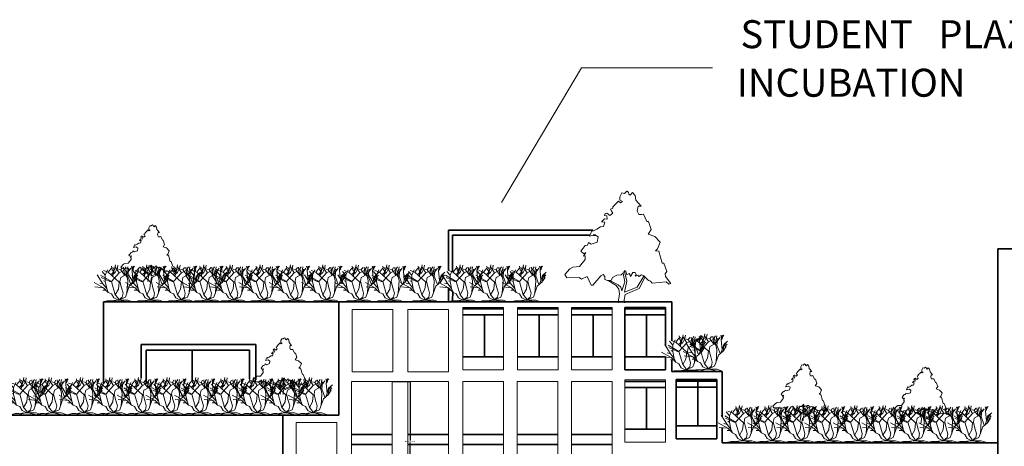
# Model space of a CAD drawing. Units: inches. Extents: x -362 to 223, y -437 to 70.
# Tile 4 of 5: x -124 to 67, y -13 to 70. Entities that reach past the tile are written whole.
import ezdxf

# ---------------------------------------------------------------- set-up
doc = ezdxf.new("R2010")
doc.units = ezdxf.units.IN
doc.header["$MEASUREMENT"] = 0
for name, color, linetype, lineweight in [('A-ANNO-DIMS', 2, 'Continuous', 18), ('A-ANNO-SYMB', 7, 'Continuous', 18), ('A-ANNO-TEXT', 7, 'Continuous', 25), ('A-ELEV', 7, 'Continuous', 35), ('A-GLAZ', 4, 'Continuous', 18), ('L-PLNT', 3, 'Continuous', 13)]:
    doc.layers.add(name, color=color, linetype=linetype, lineweight=lineweight)
doc.styles.get("Standard").update_dxf_attribs({"font": 'arial.ttf'})
doc.dimstyles.get("Standard").update_dxf_attribs({"dimtxt": 0.18, "dimasz": 0.18, "dimexe": 0.18, "dimexo": 0.0625, "dimgap": 0.09, "dimtad": 0, "dimtih": 1, "dimtoh": 1, "dimdec": 4, "dimzin": 0, "dimdsep": 46, "dimtxsty": 'Standard', "dimcen": 0.09, "dimadec": 0, "dimazin": 0, "dimtfac": 1, "dimtdec": 4, "dimtofl": 0, "dimtmove": 0, "dimatfit": 3, "dimfxl": 1, "dimtolj": 1, "dimtzin": 0, "dimarcsym": 0})

# ---------------------------------------------------------------- blocks, each defined once
blk = doc.blocks.new('*U2')
for points in [[(22.0124, 137.721), (18.5475, 141.5624), (15.5282, 138.2446), (13.8028, 139.3505), (13.3714, 142.1153), (11.2148, 143.2214), (8.1954, 140.4564), (4.7447, 141.0094), (2.1567, 136.0326), (2.1567, 131.6088), (5.6074, 129.9499), (3.0193, 128.2909), (0.4313, 130.5029), (-6.9015, 123.3141), (-6.9015, 121.6552), (-9.9208, 119.9963), (-9.0581, 118.3373), (-6.9015, 115.0195), (-10.7835, 112.2546), (-14.6656, 115.0195), (-16.8222, 114.4665), (-17.6849, 112.2546), (-14.6656, 111.7016), (-14.2342, 107.2778), (-17.6065, 107.8307), (-21.5669, 103.9599), (-17.2536, 103.4069), (-18.9789, 97.8771), (-22.8609, 97.3241), (-27.1743, 94.5593), (-32.3504, 91.7944), (-32.7817, 94.0063), (-36.6638, 85.7116), (-29.7624, 87.3705), (-25.449, 84.6056), (-26.743, 77.9699), (-34.507, 75.205), (-37.9578, 77.4169), (-39.2518, 74.099), (-42.2711, 73.5461), (-44.8592, 70.2282), (-47.8786, 66.3574), (-43.9965, 63.0395), (-41.4085, 64.6985), (-44.3346, 59.8898), (-42.2089, 60.1377), (-42.5159, 55.7849), (-49.6039, 46.4502), (-58.2307, 45.8972), (-62.1127, 43.6853), (-68.5828, 36.4966), (-65.9947, 32.0727), (-50.0352, 32.6257), (-47.0159, 30.4138), (-39.6831, 33.7317), (-34.507, 22.6721), (-32.3504, 22.6721), (-22.4296, 34.8376), (-19.4102, 36.4966), (-17.2536, 33.7317), (-17.2536, 29.8608), (-13.8028, 28.7549), (-9.0581, 28.7549), (-7.3328, 32.6257), (-1.7254, 35.3906), (3.8821, 35.9436), (6.4701, 38.1555), (6.9014, 38.7085), (8.1954, 41.4734), (9.9208, 40.3674), (11.2148, 35.9436), (14.2341, 37.6025), (15.0968, 36.4966), (15.9595, 33.7317), (18.9789, 38.7085), (21.9982, 38.7085), (23.2922, 36.4966), (21.9982, 34.2847), (25.4489, 35.3906), (26.743, 33.7317), (29.7623, 35.9436), (32.7817, 34.8376), (38.8204, 28.7549), (41.4084, 27.6489), (43.5651, 25.437), (61.6813, 27.0959), (65.132, 23.7781), (67.7201, 24.884), (60.8186, 33.7317), (60.3873, 37.0495), (62.544, 40.3674), (58.662, 50.874), (56.5053, 50.874), (52.1919, 66.3574), (47.8785, 66.9103), (50.4665, 69.1222), (53.9172, 77.9699), (47.0158, 85.1586), (38.3891, 87.9235), (42.2711, 94.0063)], [(42.2711, 94.0063), (38.8204, 104.5129), (36.6637, 104.5129), (32.3503, 113.9135), (29.7623, 113.3605), (26.743, 113.3605), (24.5862, 117.7844), (25.8802, 123.8671), (29.331, 123.8671), (22.8609, 131.6088), (21.9982, 137.6916)], [(8.1954, 40.3674), (11.2148, 27.6489), (8.1954, 13.8245), (24.5862, 19.9072), (32.7817, 34.2847)], [(-12.9401, 28.7549), (-2.588, 22.1191), (0.8626, 17.6953), (1.7253, 11.6125), (0, 0)], [(-9.9208, 28.2019), (0, 23.2251), (3.4507, 19.9072), (4.7447, 15.4834), (8.6267, 27.0959), (6.4701, 37.6025)], [(34.5071, 33.1787), (27.1743, 18.2483), (9.0581, 10.5066), (7.7641, 3.8708), (8.1954, 0)]]:
    blk.add_lwpolyline(points)
blk = doc.blocks.new('*U4')
for p, q in [((-16.8, 16.32), (-18.72, 18.72)), ((-14.88, 18.24), (-17.76, 19.2)), ((-16.8, 16.32), (-15.36, 19.68)), ((-14.88, 18.24), (-12.96, 20.64)), ((-8.16, 12), (-14.88, 18.24)), ((-13.325, 16.724), (-11.433, 18.289)), ((-12.471, 19.775), (-12.898, 22.044)), ((-11.677, 19.071), (-12.471, 19.775)), ((-11.28, 19.619), (-12.104, 21.184)), ((-12.043, 15.628), (-11.921, 18.836)), ((-11.921, 18.836), (-10.64, 20.401)), ((-11.433, 18.289), (-10.457, 22.749)), ((-10.579, 18.054), (-9.846, 19.697)), ((-8.16, 17.76), (-10.56, 21.6)), ((-9.48, 19.775), (-8.992, 22.592)), ((-7.2, 19.68), (-8.64, 20.16)), ((-8.16, 17.76), (-5.28, 19.2)), ((-7.2, 19.68), (-6.24, 21.12)), ((-4.8, 16.32), (-7.2, 19.68)), ((-5.086, 17.741), (-5.513, 21.34)), ((-5.28, 19.2), (-3.84, 21.6)), ((-2.88, 12.96), (-4.32, 19.68)), ((-3.84, 16.8), (-0.96, 20.64)), ((-3.377, 18.602), (-2.888, 21.575)), ((-2.766, 16.802), (-3.377, 18.602)), ((-2.88, 15.84), (-2.4, 20.16)), ((-0.508, 21.888), (-0.081, 20.558)), ((-0.203, 19.149), (0.102, 21.34)), ((0.346, 13.203), (-0.203, 19.149)), ((-0.142, 19.384), (0.59, 20.401)), ((-0.02, 20.01), (0.896, 21.105)), ((0.041, 20.714), (1.384, 22.044)), ((0.102, 21.34), (0.835, 21.888)), ((1.323, 16.254), (3.642, 18.289)), ((-18.24, 11.04), (-21.755, 16.655)), ((-12.96, 12.48), (-19.68, 16.32)), ((-13.92, 12.48), (-19.2, 14.88)), ((-16.8, 12.48), (-17.76, 12.96)), ((-16.8, 12.48), (-16.8, 16.32)), ((-15.84, 8.16), (-16.8, 12.48)), ((-12.96, 12.48), (-13.92, 12.48)), ((-12.96, 12.48), (-8.16, 17.76)), ((-10.56, 4.32), (-12.96, 12.48)), ((-11.982, 16.802), (-10.579, 18.054)), ((-7.68, 12.48), (-7.2, 14.88)), ((-6.72, 8.64), (-7.68, 12.48)), ((-7.2, 14.88), (-3.84, 16.8)), ((-3.377, 15.315), (-5.086, 17.819)), ((-3.36, 5.28), (-2.88, 12.96)), ((-0.96, 10.56), (-2.88, 15.84)), ((-0.48, 10.8), (0.346, 13.203)), ((0.346, 13.203), (1.323, 16.254)), ((0.96, 12), (1.44, 15.36)), ((0.96, 12), (2.88, 14.88)), ((1.44, 15.36), (2.88, 17.28)), ((1.92, 13.44), (2.4, 15.36)), ((2.4, 15.36), (3.36, 16.32)), ((-17.76, 8.64), (-23.663, 11.961)), ((-17.76, 8.64), (-23.128, 9.222)), ((-18.24, 11.04), (-20.16, 11.52)), ((-15.84, 8.16), (-18.24, 11.04)), ((-16.32, 7.2), (-18.24, 7.2)), ((-14.88, 5.76), (-17.76, 8.64)), ((-14.88, 5.76), (-15.84, 8.16)), ((-10.56, 4.32), (-8.64, 7.68)), ((-8.64, 7.68), (-8.16, 12)), ((-5.76, 5.28), (-6.72, 8.64)), ((-4.32, 2.88), (-1.92, 9.6)), ((-1.92, 9.6), (0.96, 12)), ((-15.84, 0.48), (-17.76, 0)), ((-13.44, 0.48), (-15.84, 0.48)), ((-12.96, 4.8), (-14.88, 5.76)), ((-9.6, 0.96), (-13.44, 0.48)), ((-11.52, 2.4), (-12.96, 4.8)), ((-9.6, 0.96), (-12.96, 0)), ((-8.64, 0.96), (-11.52, 2.4)), ((-8.64, 1.92), (-10.56, 4.32)), ((-9.6, 0.96), (-7.68, 0.96)), ((-8.64, 0.96), (-4.32, 2.88)), ((-8.64, 0.96), (-6.24, 2.88)), ((-8.64, 0.96), (-8.64, 1.92)), ((-8.64, 0.96), (-2.88, 0.96)), ((-7.68, 0.96), (-6.24, 0.48)), ((-6.24, 2.88), (-5.76, 5.28)), ((-6.24, 0.48), (-3.36, 0)), ((-2.88, 0.96), (0, 0))]:
    blk.add_line(p, q)
blk = doc.blocks.new('WIN-PANEL-A')
for p, q in [((0, 12.16), (7.9, 12.16)), ((0, 0), (0, 12.16)), ((7.9, 12.16), (7.9, 0)), ((7.9, 0), (0, 0))]:
    blk.add_line(p, q)
blk = doc.blocks.new('WIN-B')
for p, q in [((0, 23.36), (7.9, 23.36)), ((0, 23.36), (0, 0)), ((0, 23.36), (7.9, 23.36)), ((7.9, 0), (7.9, 23.36)), ((0, 0), (7.9, 0))]:
    blk.add_line(p, q)
blk = doc.blocks.new('*D19')
at = {"layer": 'A-ANNO-DIMS', "color": 0, "lineweight": -2, "transparency": 16777216}
for p, q in [((-51.81, 0.04), (-48.19, 0.04)), ((-48.37, -0.14), (-48.37, -11.45)), ((-48.37, -23.13), (-48.37, -11.82)), ((-51.81, -23.31), (-48.19, -23.31))]:
    blk.add_line(p, q, dxfattribs=at)
at = {"layer": 'A-ANNO-DIMS', "color": 0, "transparency": 16777216}
for points in [[(-48.4, -0.14), (-48.34, -0.14), (-48.37, 0.04)], [(-48.4, -23.13), (-48.34, -23.13), (-48.37, -23.31)]]:
    blk.add_solid(points, dxfattribs=at)
at = {"layer": 'Defpoints', "color": 0, "transparency": 16777216}
for p in [(-51.87, 0.04), (-48.37, 0.04), (-51.87, -23.31)]:
    blk.add_point(p, dxfattribs=at)
at = {"layer": 'A-ANNO-DIMS', "color": 0, "transparency": 16777216, "insert": (-48.37, -11.63), "char_height": 0.18, "attachment_point": 5}
blk.add_mtext('\\A1;WINDOW B 23 TYP.', dxfattribs=at)

msp = doc.modelspace()

# ---------------------------------------------------------------- linework, layer by layer
at = {"layer": 'A-ANNO-SYMB'}
for p, q in [((-30.56, 34.82), (-15.01, 61.06)), ((-15.01, 61.06), (10.46, 61.06))]:
    msp.add_line(p, q, dxfattribs=at)
at = {"layer": 'A-ELEV'}
for p, q in [((-40.87, 29.45), (-12.83, 29.45)), ((-40.87, 21.6), (-40.87, 29.45)), ((-40.13, 28.49), (-13.37, 28.49)), ((-40.13, 21.35), (-40.13, 28.49)), ((-12.78, 28.49), (-12.26, 28.49)), ((65.97, 25.83), (120.64, 25.83)), ((65.97, 25.83), (65.97, -1.59)), ((-40.89, 15.55), (-40.89, 18.27)), ((-40.08, 15.7), (-40.05, 17.54)), ((-62.22, 15.55), (-107.98, 15.55)), ((-107.98, 15.55), (-107.98, -0.39)), ((2.55, 15.55), (-62.22, 15.55)), ((-62.22, 15.55), (-62.22, -6.5)), ((-40.87, 15.55), (-40.87, 15.55)), ((2.55, 15.55), (-0.43, 15.55)), ((2.55, 7.97), (2.55, 15.55)), ((-38.11, 14.14), (-30.21, 14.14)), ((-27.44, 14.14), (-19.54, 14.14)), ((-16.98, 14.14), (-9.08, 14.14)), ((-6.6, 14.46), (1.3, 14.46)), ((-6.6, 2.3), (-6.6, 14.46)), ((-6.6, 14.14), (1.3, 14.14)), ((1.3, 14.46), (1.3, 6.99)), ((-38.11, 12.98), (-30.21, 12.98)), ((-33.9, 4.84), (-33.9, 12.98)), ((-27.44, 12.98), (-19.54, 12.98)), ((-23.24, 4.84), (-23.24, 12.98)), ((-16.98, 12.98), (-9.08, 12.98)), ((-12.77, 4.84), (-12.77, 12.98)), ((-6.6, 12.98), (1.3, 12.98)), ((-2.4, 4.84), (-2.4, 12.98)), ((-100.68, 0.76), (-100.68, 7.25)), ((-100.68, 7.25), (-78.35, 7.25)), ((-99.66, 6.16), (-79.56, 6.16)), ((-99.66, -0.38), (-99.66, 6.16)), ((-90.72, 0.11), (-90.72, 6.16)), ((-79.56, 0.59), (-79.56, 6.16)), ((-78.35, 7.25), (-78.35, 0.38)), ((-38.11, 4.84), (-30.21, 4.84)), ((-27.44, 4.84), (-19.54, 4.84)), ((-16.98, 4.84), (-9.08, 4.84)), ((-6.6, 4.84), (1.3, 4.84)), ((1.3, 4.84), (1.3, 2.3)), ((2.55, 2.01), (2.55, 4.23)), ((1.3, 2.3), (-6.6, 2.3)), ((12.37, 2.01), (2.55, 2.01)), ((12.37, 0.45), (12.37, 2.01)), ((-6.6, 0.06), (1.3, 0.06)), ((11.28, 0.45), (3.37, 0.45)), ((3.37, -11.12), (3.37, 0.45)), ((3.37, 0.09), (11.28, 0.09)), ((7.58, -8.58), (7.58, 0.09)), ((11.28, 0.45), (11.28, -11.12)), ((12.37, -6.85), (12.37, 0.45)), ((-6.6, -1.1), (1.3, -1.1)), ((-2.4, -9.25), (-2.4, -1.1)), ((3.4, -1.06), (11.28, -1.06)), ((65.97, -1.59), (65.97, -5.1)), ((-107.98, -2.18), (-107.98, -2.37)), ((65.97, -5.1), (65.97, -11.87)), ((-62.22, -6.5), (-142.63, -6.5)), ((-107.98, -6.2), (-107.98, -6.5)), ((-73.12, -6.5), (-73.12, -25.79)), ((65.97, -6.52), (65.97, -6.62)), ((-6.6, -9.25), (1.3, -9.25)), ((3.37, -8.58), (11.28, -8.58)), ((12.37, -11.87), (12.37, -8.94)), ((-59.77, -10.28), (-51.87, -10.28)), ((-48.8, -10.28), (-40.9, -10.28)), ((-38.09, -10.28), (-30.19, -10.28)), ((-27.52, -10.28), (-19.61, -10.28)), ((-16.94, -10.28), (-9.04, -10.28)), ((11.28, -11.12), (3.37, -11.12)), ((-59.77, -12.2), (-51.87, -12.2)), ((-48.8, -12.2), (-40.9, -12.2)), ((-38.09, -12.2), (-30.19, -12.2)), ((-27.52, -12.2), (-19.61, -12.2)), ((-16.94, -12.2), (-9.04, -12.2)), ((65.97, -11.87), (12.37, -11.87)), ((65.97, -11.74), (65.97, -58.78))]:
    msp.add_line(p, q, dxfattribs=at)

# ---------------------------------------------------------------- block references
at = {"layer": 'A-GLAZ', "rotation": 180}
for p in [(-51.74, 14.06), (-40.87, 14.06), (-30.21, 14.46), (-19.54, 14.46), (-9.08, 14.46), (1.3, 0.38), (-62.63, -7.93)]:
    msp.add_blockref('WIN-PANEL-A', p, dxfattribs=at)
at = {"layer": 'A-GLAZ'}
for p in [(-59.77, -23.31), (-48.8, -23.31), (-38.09, -23.31), (-27.52, -23.31), (-16.94, -23.31)]:
    msp.add_blockref('WIN-B', p, dxfattribs=at)
at = {"layer": 'L-PLNT'}
for name, p, xscale, yscale, zscale in [('*U2', (-7.89, 15.34), 0.1515196865409096, 0.1515196865409096, 0.1515196865409096), ('*U2', (-99.34, 19.48), 0.0769249465327344, 0.0769249465327344, 0.0769249465327344), ('*U4', (-102.36, 15.55), 0.3151431067188808, 0.3151431067188808, 0.3151431067188808), ('*U4', (-96.24, 15.55), 0.3151431067188808, 0.3151431067188808, 0.3151431067188808), ('*U4', (-90.26, 15.55), 0.3151431067188808, 0.3151431067188808, 0.3151431067188808), ('*U4', (-85.15, 15.55), 0.3151431067188808, 0.3151431067188808, 0.3151431067188808), ('*U4', (-80.03, 15.55), 0.3151431067188808, 0.3151431067188808, 0.3151431067188808), ('*U4', (-74.21, 15.55), 0.3151431067188808, 0.3151431067188808, 0.3151431067188808), ('*U4', (-68.31, 15.55), 0.3151431067188808, 0.3151431067188808, 0.3151431067188808), ('*U4', (-62.02, 15.55), 0.3151431067188808, 0.3151431067188808, 0.3151431067188808), ('*U4', (-55.57, 15.55), 0.3151431067188808, 0.3151431067188808, 0.3151431067188808), ('*U4', (-49.59, 15.55), 0.3151431067188808, 0.3151431067188808, 0.3151431067188808), ('*U4', (-42.74, 15.55), 0.3151431067188808, 0.3151431067188808, 0.3151431067188808), ('*U4', (-35.29, 15.55), 0.3151431067188808, 0.3151431067188808, 0.3151431067188808), ('*U4', (-29.37, 15.55), 0.3151431067188808, 0.3151431067188808, 0.3151431067188808), ('*U4', (-23.01, 15.55), 0.3151431067188808, 0.3151431067188808, 0.3151431067188808), ('*U2', (-73.65, -2.48), 0.0769249465327344, 0.0769249465327344, 0.0769249465327344), ('*U4', (8.02, 1.96), 0.3151431067188808, 0.3151431067188808, 0.3151431067188808), ('*U4', (12.24, 2.13), 0.3151431067188808, 0.3151431067188808, 0.3151431067188808), ('*U2', (27.49, -7.57), 0.0769249465327344, 0.0769249465327344, 0.0769249465327344), ('*U2', (51, -8.17), 0.0769249465327344, 0.0769249465327344, 0.0769249465327344), ('*U4', (-120.18, -6.36), 0.3151431067188808, 0.3151431067188808, 0.3151431067188808), ('*U4', (-115.26, -6.36), 0.3151431067188808, 0.3151431067188808, 0.3151431067188808), ('*U4', (-109.17, -6.36), 0.3151431067188808, 0.3151431067188808, 0.3151431067188808), ('*U4', (-103.46, -6.36), 0.3151431067188808, 0.3151431067188808, 0.3151431067188808), ('*U4', (-97.85, -6.36), 0.3151431067188808, 0.3151431067188808, 0.3151431067188808), ('*U4', (-92.31, -6.36), 0.3151431067188808, 0.3151431067188808, 0.3151431067188808), ('*U4', (-86.74, -6.36), 0.3151431067188808, 0.3151431067188808, 0.3151431067188808), ('*U4', (-81.09, -6.36), 0.3151431067188808, 0.3151431067188808, 0.3151431067188808), ('*U4', (-75.5, -6.36), 0.3151431067188808, 0.3151431067188808, 0.3151431067188808), ('*U4', (-69.95, -6.36), 0.3151431067188808, 0.3151431067188808, 0.3151431067188808), ('*U4', (-64.61, -6.36), 0.3151431067188808, 0.3151431067188808, 0.3151431067188808), ('*U4', (19.03, -11.78), 0.3151431067188808, 0.3151431067188808, 0.3151431067188808), ('*U4', (24.71, -11.78), 0.3151431067188808, 0.3151431067188808, 0.3151431067188808), ('*U4', (30.25, -11.78), 0.3151431067188808, 0.3151431067188808, 0.3151431067188808), ('*U4', (35.79, -11.78), 0.3151431067188808, 0.3151431067188808, 0.3151431067188808), ('*U4', (41.41, -11.78), 0.3151431067188808, 0.3151431067188808, 0.3151431067188808), ('*U4', (46.93, -11.78), 0.3151431067188808, 0.3151431067188808, 0.3151431067188808), ('*U4', (52.54, -11.78), 0.3151431067188808, 0.3151431067188808, 0.3151431067188808), ('*U4', (58.04, -11.78), 0.3151431067188808, 0.3151431067188808, 0.3151431067188808), ('*U4', (63.62, -11.78), 0.3151431067188808, 0.3151431067188808, 0.3151431067188808)]:
    msp.add_blockref(name, p, dxfattribs=dict(at, xscale=xscale, yscale=yscale, zscale=zscale))

# ---------------------------------------------------------------- texts
at = {"layer": 'A-ANNO-TEXT'}
for s, height, p in [('STUDENT   PLAZA', 5.4377, (15.9, 64.85)), ('INCUBATION', 5.438, (15.17, 55.41))]:
    msp.add_text(s, height=height, dxfattribs=at).set_placement(p)

# ---------------------------------------------------------------- dimensions: what is measured, and where the dimension line sits
at = {"layer": 'A-ANNO-DIMS'}
dim = msp.add_linear_dim(base=(-48.37, 0.04), p1=(-51.87, -23.31), p2=(-51.87, 0.04), angle=90, text='WINDOW B <> TYP.', dimstyle='Standard', override={"dimdec": 0, "dimlfac": 1, "dimrnd": 0, "dimzin": 0, "dimdsep": 46, "dimlunit": 2}, dxfattribs=at)
dim.commit()
dim.dimension.update_dxf_attribs({"geometry": '*D19', "text_midpoint": (-48.37, -11.63)})

doc.saveas('drawing.dxf')
